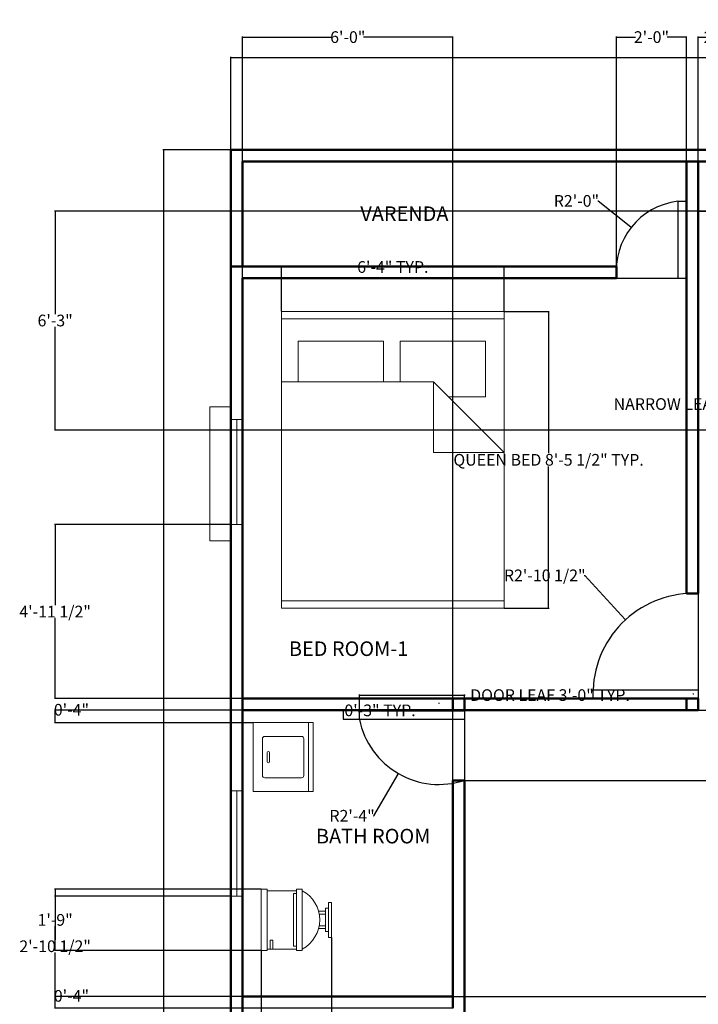
# Model space of a CAD drawing. Units: inches. Extents: x 749 to 1356, y 222 to 907.
# Tile 3 of 4: x 749 to 981, y 570 to 907. Entities that reach past the tile are written whole.
import ezdxf

# ---------------------------------------------------------------- set-up
doc = ezdxf.new("R2010")
doc.units = ezdxf.units.IN
doc.header["$MEASUREMENT"] = 0
for name, color, linetype, lineweight in [('A-ANNO-DIMS', 30, 'Continuous', 18), ('A-AREA-IDEN', 6, 'Continuous', 25), ('A-FLOR-CASE', 34, 'Continuous', 25), ('A-FLOR-FIXT', 9, 'Continuous', 18), ('A-GLAZ', 4, 'Continuous', 20), ('A-WALL', 7, 'Continuous', 50), ('DOOR', 4, 'Continuous', 25), ('FURNITURE', 32, 'Continuous', 18)]:
    doc.layers.add(name, color=color, linetype=linetype, lineweight=lineweight)
doc.styles.get("Standard").update_dxf_attribs({"font": 'arial.ttf'})
doc.dimstyles.get("Standard").update_dxf_attribs({"dimtxt": 4, "dimasz": 0.18, "dimexe": 0.18, "dimexo": 0.0625, "dimgap": 0.09, "dimtad": 0, "dimtih": 1, "dimtoh": 1, "dimdec": 0, "dimrnd": 6, "dimzin": 0, "dimdsep": 46, "dimlunit": 3, "dimtxsty": 'Standard', "dimcen": 0.09, "dimadec": 0, "dimazin": 0, "dimtfac": 1, "dimtdec": 0, "dimtofl": 0, "dimtmove": 0, "dimatfit": 3, "dimfxl": 1, "dimtolj": 1, "dimtzin": 0, "dimarcsym": 0})

# ---------------------------------------------------------------- blocks, each defined once
blk = doc.blocks.new('Toilet - Imperial')
for p, q in [((-10, 22), (-10, 12)), ((-10, 21), (-7, 21)), ((-7, 21), (-7, 20)), ((10, 12), (10, 22)), ((-7, 20), (-10, 20)), ((10.5, 12), (-10.5, 12)), ((-10.5, 10), (-10.5, 12)), ((9, 13), (-9, 13)), ((-9, 13), (-9, 12)), ((9, 12), (9, 13)), ((10.5, 12), (10.5, 10)), ((10.5, 10), (-10.5, 10)), ((-3, 4.4065), (-3, 2)), ((-2, 2), (-2, 4.1658)), ((2, 4.1658), (2, 2)), ((3, 2), (3, 4.4065)), ((4, 2), (-4, 2)), ((-4, 2), (-4, 1)), ((4, 1), (4, 2))]:
    blk.add_line(p, q)
for points in [[(10.5, 22), (10.5, 24), (-10.5, 24), (-10.5, 22)], [(6, 0), (6, 1), (-6, 1), (-6, 0)]]:
    blk.add_lwpolyline(points, close=True)
blk.add_arc((0, 15.3333), 11.3333, 208.0725, 331.9275)
blk = doc.blocks.new('QUEEN-00')
for p, q in [((-0.8475, -0.7751), (-0.8475, 0.7489)), ((0.6511, 0.7489), (0.6511, -0.2925)), ((1.0829, 0.7489), (1.0829, -0.7751)), ((0.9305, 0.6346), (0.6511, 0.6346)), ((0.9305, 0.0504), (0.9305, 0.6346)), ((0.6511, 0.0504), (0.9305, 0.0504)), ((0.9305, -0.0639), (0.6511, -0.0639)), ((0.9305, -0.6481), (0.9305, -0.0639)), ((0.1685, -0.7751), (0.6511, -0.2925)), ((0.1685, -0.2925), (0.1685, -0.7751)), ((0.6511, -0.2925), (0.1685, -0.2925)), ((0.5495, -0.3941), (0.5495, -0.6481)), ((0.5495, -0.6481), (0.9305, -0.6481))]:
    blk.add_line(p, q)
blk.add_lwpolyline([(-0.8983, -0.7751), (-0.8983, 0.7489), (1.1337, 0.7489), (1.1337, -0.7751)], close=True)
blk = doc.blocks.new('LAVAD-01')
for p, q in [((-0.322, 0.358), (-0.322, -0.392)), ((0.328, 0.358), (-0.322, 0.358)), ((-0.272, 0.358), (-0.272, -0.392)), ((0.328, -0.392), (0.328, 0.358)), ((-0.222, 0.183), (-0.222, -0.217)), ((0.203, 0.208), (-0.197, 0.208)), ((0.228, -0.217), (0.228, 0.183)), ((0.153, 0.033), (0.153, -0.067)), ((0.165, 0.046), (0.165, 0.046)), ((0.178, -0.067), (0.178, 0.033)), ((0.165, -0.079), (0.165, -0.079)), ((-0.197, -0.242), (0.203, -0.242)), ((-0.322, -0.392), (0.328, -0.392))]:
    blk.add_line(p, q)
for centre, radius, start, end in [((-0.197, 0.183), 0.025, 90, 180), ((0.203, 0.183), 0.025, 0, 90), ((0.165, 0.033), 0.0125, 90, 180), ((0.165, 0.033), 0.0125, 0, 90), ((0.165, -0.067), 0.0125, 180, 270), ((0.165, -0.067), 0.0125, 270, 360), ((-0.197, -0.217), 0.025, 180, 270), ((0.203, -0.217), 0.025, 270, 360)]:
    blk.add_arc(centre, radius, start, end)
blk = doc.blocks.new('*D129')
at = {"layer": 'A-ANNO-DIMS', "color": 0, "lineweight": -2, "transparency": 16777216}
for p, q in [((820.88, 858.33), (820.88, 894.09)), ((821.06, 893.91), (1057.31, 893.91)), ((1300.7, 893.91), (1064.44, 893.91)), ((1300.88, 862.33), (1300.88, 894.09))]:
    blk.add_line(p, q, dxfattribs=at)
at = {"layer": 'A-ANNO-DIMS', "color": 0, "transparency": 16777216}
for points in [[(821.06, 893.94), (821.06, 893.88), (820.88, 893.91)], [(1300.7, 893.94), (1300.7, 893.88), (1300.88, 893.91)]]:
    blk.add_solid(points, dxfattribs=at)
at = {"layer": 'Defpoints', "color": 0, "transparency": 16777216}
for p in [(1300.88, 893.91), (1300.88, 862.27), (820.88, 858.27)]:
    blk.add_point(p, dxfattribs=at)
at = {"layer": 'A-ANNO-DIMS', "color": 0, "transparency": 16777216, "insert": (1060.88, 893.91), "char_height": 4, "attachment_point": 5}
blk.add_mtext("\\A1;40'", dxfattribs=at)
blk = doc.blocks.new('*D130')
at = {"layer": 'A-ANNO-DIMS', "color": 0, "lineweight": -2, "transparency": 16777216}
for p, q in [((820.81, 862.27), (797.55, 862.27)), ((797.73, 862.09), (797.73, 564.4)), ((797.73, 262.45), (797.73, 560.13)), ((820.81, 262.27), (797.55, 262.27))]:
    blk.add_line(p, q, dxfattribs=at)
at = {"layer": 'A-ANNO-DIMS', "color": 0, "transparency": 16777216}
for points in [[(797.7, 862.09), (797.76, 862.09), (797.73, 862.27)], [(797.7, 262.45), (797.76, 262.45), (797.73, 262.27)]]:
    blk.add_solid(points, dxfattribs=at)
at = {"layer": 'Defpoints', "color": 0, "transparency": 16777216}
for p in [(820.88, 862.27), (797.73, 262.27), (820.88, 262.27)]:
    blk.add_point(p, dxfattribs=at)
at = {"layer": 'A-ANNO-DIMS', "color": 0, "transparency": 16777216, "insert": (797.73, 562.27), "char_height": 4, "attachment_point": 5}
blk.add_mtext("\\A1;50'", dxfattribs=at)
blk = doc.blocks.new('WIN-36IN')
blk.add_lwpolyline([(0, 0), (0, 36), (4, 36), (4, 0)], close=True)
blk.add_lwpolyline([(4, 0), (2.02, 0), (2.02, 36)])
blk = doc.blocks.new('DOOR-LEAF-36IN')
blk.add_lwpolyline([(0, 3), (36, 3), (36, 0), (0, 0)], close=True)
blk = doc.blocks.new('*D137')
at = {"layer": 'A-ANNO-DIMS', "color": 0, "lineweight": -2, "transparency": 16777216}
for p, q in [((864.87, 670.13), (864.87, 675.65)), ((865.05, 675.47), (900.69, 675.47)), ((900.87, 670.13), (900.87, 675.65)), ((900.87, 675.47), (901.05, 675.47))]:
    blk.add_line(p, q, dxfattribs=at)
at = {"layer": 'A-ANNO-DIMS', "color": 0, "transparency": 16777216}
for points in [[(865.05, 675.5), (865.05, 675.44), (864.87, 675.47)], [(900.69, 675.5), (900.69, 675.44), (900.87, 675.47)]]:
    blk.add_solid(points, dxfattribs=at)
at = {"layer": 'Defpoints', "color": 0, "transparency": 16777216}
for p in [(900.87, 675.47), (864.87, 670.07), (900.87, 670.07)]:
    blk.add_point(p, dxfattribs=at)
at = {"layer": 'A-ANNO-DIMS', "color": 0, "transparency": 16777216, "insert": (930.15, 675.47), "char_height": 4, "attachment_point": 5}
blk.add_mtext('\\A1;DOOR LEAF 3\'-0" TYP.', dxfattribs=at)
blk = doc.blocks.new('*D138')
at = {"layer": 'A-ANNO-DIMS', "color": 0, "lineweight": -2, "transparency": 16777216}
for p, q in [((864.81, 670.07), (859.29, 670.07)), ((859.47, 670.07), (859.47, 670.25)), ((859.47, 670.25), (859.65, 670.25)), ((859.47, 667.25), (859.47, 669.89)), ((864.81, 667.07), (859.29, 667.07))]:
    blk.add_line(p, q, dxfattribs=at)
at = {"layer": 'A-ANNO-DIMS', "color": 0, "transparency": 16777216}
for points in [[(859.44, 669.89), (859.5, 669.89), (859.47, 670.07)], [(859.44, 667.25), (859.5, 667.25), (859.47, 667.07)]]:
    blk.add_solid(points, dxfattribs=at)
at = {"layer": 'Defpoints', "color": 0, "transparency": 16777216}
for p in [(859.47, 670.07), (864.87, 670.07), (864.87, 667.07)]:
    blk.add_point(p, dxfattribs=at)
at = {"layer": 'A-ANNO-DIMS', "color": 0, "transparency": 16777216, "insert": (871.93, 670.25), "char_height": 4, "attachment_point": 5}
blk.add_mtext('\\A1;0\'-3" TYP.', dxfattribs=at)
blk = doc.blocks.new('*D141')
at = {"layer": 'A-ANNO-DIMS', "color": 0, "lineweight": -2, "transparency": 16777216}
for p, q in [((984.05, 787.99), (988.01, 787.99)), ((987.83, 787.81), (987.83, 777.32)), ((987.83, 762.5), (987.83, 773)), ((984.05, 762.32), (988.01, 762.32))]:
    blk.add_line(p, q, dxfattribs=at)
at = {"layer": 'A-ANNO-DIMS', "color": 0, "transparency": 16777216}
for points in [[(987.8, 787.81), (987.86, 787.81), (987.83, 787.99)], [(987.8, 762.5), (987.86, 762.5), (987.83, 762.32)]]:
    blk.add_solid(points, dxfattribs=at)
at = {"layer": 'Defpoints', "color": 0, "transparency": 16777216}
for p in [(983.98, 787.99), (987.83, 787.99), (983.98, 762.32)]:
    blk.add_point(p, dxfattribs=at)
at = {"layer": 'A-ANNO-DIMS', "color": 0, "transparency": 16777216, "insert": (987.83, 775.16), "char_height": 4, "attachment_point": 5}
blk.add_mtext('\\A1;NARROW LEAF 2\'-1 1/2" TYP.', dxfattribs=at)
blk = doc.blocks.new('*D147')
at = {"layer": 'A-ANNO-DIMS', "color": 0, "lineweight": -2, "transparency": 16777216}
for p, q in [((914.47, 806.86), (929.83, 806.86)), ((929.65, 806.68), (929.65, 758.35)), ((929.65, 705.44), (929.65, 753.78)), ((914.47, 705.26), (929.83, 705.26))]:
    blk.add_line(p, q, dxfattribs=at)
at = {"layer": 'A-ANNO-DIMS', "color": 0, "transparency": 16777216}
for points in [[(929.62, 806.68), (929.68, 806.68), (929.65, 806.86)], [(929.62, 705.44), (929.68, 705.44), (929.65, 705.26)]]:
    blk.add_solid(points, dxfattribs=at)
at = {"layer": 'Defpoints', "color": 0, "transparency": 16777216}
for p in [(914.41, 806.86), (929.65, 806.86), (914.41, 705.26)]:
    blk.add_point(p, dxfattribs=at)
at = {"layer": 'A-ANNO-DIMS', "color": 0, "transparency": 16777216, "insert": (929.65, 756.06), "char_height": 4, "attachment_point": 5}
blk.add_mtext('\\A1;QUEEN BED 8\'-5 1/2" TYP.', dxfattribs=at)
blk = doc.blocks.new('*D148')
at = {"layer": 'A-ANNO-DIMS', "color": 0, "lineweight": -2, "transparency": 16777216}
for p, q in [((838.21, 806.93), (838.21, 822.28)), ((838.39, 822.1), (864.02, 822.1)), ((914.23, 822.1), (888.6, 822.1)), ((914.41, 806.93), (914.41, 822.28))]:
    blk.add_line(p, q, dxfattribs=at)
at = {"layer": 'A-ANNO-DIMS', "color": 0, "transparency": 16777216}
for points in [[(838.39, 822.13), (838.39, 822.07), (838.21, 822.1)], [(914.23, 822.13), (914.23, 822.07), (914.41, 822.1)]]:
    blk.add_solid(points, dxfattribs=at)
at = {"layer": 'Defpoints', "color": 0, "transparency": 16777216}
for p in [(838.21, 822.1), (838.21, 806.86), (914.41, 806.86)]:
    blk.add_point(p, dxfattribs=at)
at = {"layer": 'A-ANNO-DIMS', "color": 0, "transparency": 16777216, "insert": (876.31, 822.1), "char_height": 4, "attachment_point": 5}
blk.add_mtext('\\A1;6\'-4" TYP.', dxfattribs=at)
blk = doc.blocks.new('*D167')
at = {"layer": 'A-ANNO-DIMS', "color": 0, "lineweight": -2, "transparency": 16777216}
for p, q in [((820.83, 733.87), (760.48, 733.87)), ((760.66, 733.69), (760.66, 706.22)), ((760.66, 674.45), (760.66, 701.91)), ((824.81, 674.27), (760.48, 674.27))]:
    blk.add_line(p, q, dxfattribs=at)
at = {"layer": 'A-ANNO-DIMS', "color": 0, "transparency": 16777216}
for points in [[(760.63, 733.69), (760.69, 733.69), (760.66, 733.87)], [(760.63, 674.45), (760.69, 674.45), (760.66, 674.27)]]:
    blk.add_solid(points, dxfattribs=at)
at = {"layer": 'Defpoints', "color": 0, "transparency": 16777216}
for p in [(760.66, 733.87), (820.89, 733.87), (824.88, 674.27)]:
    blk.add_point(p, dxfattribs=at)
at = {"layer": 'A-ANNO-DIMS', "color": 0, "transparency": 16777216, "insert": (760.66, 704.07), "char_height": 4, "attachment_point": 5}
blk.add_mtext('\\A1;4\'-11 1/2"', dxfattribs=at)
blk = doc.blocks.new('*D169')
at = {"layer": 'A-ANNO-DIMS', "color": 0, "lineweight": -2, "transparency": 16777216}
for p, q in [((980.88, 858.33), (980.88, 901.02)), ((981.06, 900.84), (997, 900.84)), ((1033.23, 900.84), (1017.29, 900.84)), ((1033.41, 858.31), (1033.41, 901.02))]:
    blk.add_line(p, q, dxfattribs=at)
at = {"layer": 'A-ANNO-DIMS', "color": 0, "transparency": 16777216}
for points in [[(981.06, 900.87), (981.06, 900.81), (980.88, 900.84)], [(1033.23, 900.87), (1033.23, 900.81), (1033.41, 900.84)]]:
    blk.add_solid(points, dxfattribs=at)
at = {"layer": 'Defpoints', "color": 0, "transparency": 16777216}
for p in [(1033.41, 900.84), (980.88, 858.27), (1033.41, 858.25)]:
    blk.add_point(p, dxfattribs=at)
at = {"layer": 'A-ANNO-DIMS', "color": 0, "transparency": 16777216, "insert": (1007.14, 900.84), "char_height": 4, "attachment_point": 5}
blk.add_mtext('\\A1;4\'-4 1/2"', dxfattribs=at)
blk = doc.blocks.new('*D171')
at = {"layer": 'A-ANNO-DIMS', "color": 0, "lineweight": -2, "transparency": 16777216}
for p, q in [((820.81, 606.63), (760.48, 606.63)), ((760.66, 606.45), (760.66, 591.61)), ((760.66, 572.45), (760.66, 587.29)), ((824.81, 572.27), (760.48, 572.27))]:
    blk.add_line(p, q, dxfattribs=at)
at = {"layer": 'A-ANNO-DIMS', "color": 0, "transparency": 16777216}
for points in [[(760.63, 606.45), (760.69, 606.45), (760.66, 606.63)], [(760.63, 572.45), (760.69, 572.45), (760.66, 572.27)]]:
    blk.add_solid(points, dxfattribs=at)
at = {"layer": 'Defpoints', "color": 0, "transparency": 16777216}
for p in [(760.66, 606.63), (820.87, 606.63), (824.88, 572.27)]:
    blk.add_point(p, dxfattribs=at)
at = {"layer": 'A-ANNO-DIMS', "color": 0, "transparency": 16777216, "insert": (760.66, 589.45), "char_height": 4, "attachment_point": 5}
blk.add_mtext('\\A1;2\'-10 1/2"', dxfattribs=at)
blk = doc.blocks.new('*D172')
at = {"layer": 'A-ANNO-DIMS', "color": 0, "lineweight": -2, "transparency": 16777216}
for p, q in [((824.88, 572.33), (824.88, 901.02)), ((825.06, 900.84), (855.46, 900.84)), ((896.7, 900.84), (866.29, 900.84)), ((896.88, 572.33), (896.88, 901.02))]:
    blk.add_line(p, q, dxfattribs=at)
at = {"layer": 'A-ANNO-DIMS', "color": 0, "transparency": 16777216}
for points in [[(825.06, 900.87), (825.06, 900.81), (824.88, 900.84)], [(896.7, 900.87), (896.7, 900.81), (896.88, 900.84)]]:
    blk.add_solid(points, dxfattribs=at)
at = {"layer": 'Defpoints', "color": 0, "transparency": 16777216}
for p in [(896.88, 900.84), (824.88, 572.27), (896.88, 572.27)]:
    blk.add_point(p, dxfattribs=at)
at = {"layer": 'A-ANNO-DIMS', "color": 0, "transparency": 16777216, "insert": (860.88, 900.84), "char_height": 4, "attachment_point": 5}
blk.add_mtext('\\A1;6\'-0"', dxfattribs=at)
blk = doc.blocks.new('*D174')
at = {"layer": 'A-ANNO-DIMS', "color": 0, "lineweight": -2, "transparency": 16777216}
for p, q in [((900.94, 646.27), (1340.58, 646.27)), ((1340.4, 646.09), (1340.4, 611.4)), ((1340.4, 572.45), (1340.4, 607.13)), ((896.94, 572.27), (1340.58, 572.27))]:
    blk.add_line(p, q, dxfattribs=at)
at = {"layer": 'A-ANNO-DIMS', "color": 0, "transparency": 16777216}
for points in [[(1340.37, 646.09), (1340.43, 646.09), (1340.4, 646.27)], [(1340.37, 572.45), (1340.43, 572.45), (1340.4, 572.27)]]:
    blk.add_solid(points, dxfattribs=at)
at = {"layer": 'Defpoints', "color": 0, "transparency": 16777216}
for p in [(900.88, 646.27), (1340.4, 646.27), (896.88, 572.27)]:
    blk.add_point(p, dxfattribs=at)
at = {"layer": 'A-ANNO-DIMS', "color": 0, "transparency": 16777216, "insert": (1340.4, 609.27), "char_height": 4, "attachment_point": 5}
blk.add_mtext('\\A1;6\'-2"', dxfattribs=at)
blk = doc.blocks.new('*D175')
at = {"layer": 'A-ANNO-DIMS', "color": 0, "lineweight": -2, "transparency": 16777216}
for p, q in [((900.94, 670.27), (1340.58, 670.27)), ((1340.4, 670.09), (1340.4, 660.4)), ((1340.4, 646.45), (1340.4, 656.13)), ((900.94, 646.27), (1340.58, 646.27))]:
    blk.add_line(p, q, dxfattribs=at)
at = {"layer": 'A-ANNO-DIMS', "color": 0, "transparency": 16777216}
for points in [[(1340.37, 670.09), (1340.43, 670.09), (1340.4, 670.27)], [(1340.37, 646.45), (1340.43, 646.45), (1340.4, 646.27)]]:
    blk.add_solid(points, dxfattribs=at)
at = {"layer": 'Defpoints', "color": 0, "transparency": 16777216}
for p in [(900.88, 670.27), (1340.4, 670.27), (900.88, 646.27)]:
    blk.add_point(p, dxfattribs=at)
at = {"layer": 'A-ANNO-DIMS', "color": 0, "transparency": 16777216, "insert": (1340.4, 658.27), "char_height": 4, "attachment_point": 5}
blk.add_mtext('\\A1;2\'-0"', dxfattribs=at)
blk = doc.blocks.new('*D177')
at = {"layer": 'A-ANNO-DIMS', "color": 0, "lineweight": -2, "transparency": 16777216}
for p, q in [((855.27, 592.42), (855.27, 224.8)), ((831.27, 587.92), (831.27, 224.8)), ((831.45, 224.98), (837.83, 224.98)), ((855.09, 224.98), (848.71, 224.98))]:
    blk.add_line(p, q, dxfattribs=at)
at = {"layer": 'A-ANNO-DIMS', "color": 0, "transparency": 16777216}
for points in [[(831.45, 225.01), (831.45, 224.95), (831.27, 224.98)], [(855.09, 225.01), (855.09, 224.95), (855.27, 224.98)]]:
    blk.add_solid(points, dxfattribs=at)
at = {"layer": 'Defpoints', "color": 0, "transparency": 16777216}
for p in [(855.27, 592.48), (831.27, 587.98), (855.27, 224.98)]:
    blk.add_point(p, dxfattribs=at)
at = {"layer": 'A-ANNO-DIMS', "color": 0, "transparency": 16777216, "insert": (843.27, 224.98), "char_height": 4, "attachment_point": 5}
blk.add_mtext('\\A1;2\'-0"', dxfattribs=at)
blk = doc.blocks.new('*D178')
at = {"layer": 'A-ANNO-DIMS', "color": 0, "lineweight": -2, "transparency": 16777216}
for p, q in [((831.21, 608.98), (760.48, 608.98)), ((760.66, 608.8), (760.66, 600.62)), ((760.66, 588.16), (760.66, 596.35)), ((831.21, 587.98), (760.48, 587.98))]:
    blk.add_line(p, q, dxfattribs=at)
at = {"layer": 'A-ANNO-DIMS', "color": 0, "transparency": 16777216}
for points in [[(760.63, 608.8), (760.69, 608.8), (760.66, 608.98)], [(760.63, 588.16), (760.69, 588.16), (760.66, 587.98)]]:
    blk.add_solid(points, dxfattribs=at)
at = {"layer": 'Defpoints', "color": 0, "transparency": 16777216}
for p in [(760.66, 608.98), (831.27, 608.98), (831.27, 587.98)]:
    blk.add_point(p, dxfattribs=at)
at = {"layer": 'A-ANNO-DIMS', "color": 0, "transparency": 16777216, "insert": (760.66, 598.48), "char_height": 4, "attachment_point": 5}
blk.add_mtext('\\A1;1\'-9"', dxfattribs=at)
blk = doc.blocks.new('*D179')
at = {"layer": 'A-ANNO-DIMS', "color": 0, "lineweight": -2, "transparency": 16777216}
for p, q in [((1112.81, 841.27), (760.48, 841.27)), ((760.66, 841.09), (760.66, 805.9)), ((760.66, 766.45), (760.66, 801.63)), ((1112.81, 766.27), (760.48, 766.27))]:
    blk.add_line(p, q, dxfattribs=at)
at = {"layer": 'A-ANNO-DIMS', "color": 0, "transparency": 16777216}
for points in [[(760.63, 841.09), (760.69, 841.09), (760.66, 841.27)], [(760.63, 766.45), (760.69, 766.45), (760.66, 766.27)]]:
    blk.add_solid(points, dxfattribs=at)
at = {"layer": 'Defpoints', "color": 0, "transparency": 16777216}
for p in [(760.66, 841.27), (1112.88, 841.27), (1112.88, 766.27)]:
    blk.add_point(p, dxfattribs=at)
at = {"layer": 'A-ANNO-DIMS', "color": 0, "transparency": 16777216, "insert": (760.66, 803.77), "char_height": 4, "attachment_point": 5}
blk.add_mtext('\\A1;6\'-3"', dxfattribs=at)
blk = doc.blocks.new('*D182')
at = {"layer": 'A-ANNO-DIMS', "color": 0, "lineweight": -2, "transparency": 16777216}
for p, q in [((980.94, 858.27), (1340.58, 858.27)), ((1340.4, 858.09), (1340.4, 851.9)), ((1340.4, 841.45), (1340.4, 847.63)), ((980.94, 841.27), (1340.58, 841.27))]:
    blk.add_line(p, q, dxfattribs=at)
at = {"layer": 'A-ANNO-DIMS', "color": 0, "transparency": 16777216}
for points in [[(1340.37, 858.09), (1340.43, 858.09), (1340.4, 858.27)], [(1340.37, 841.45), (1340.43, 841.45), (1340.4, 841.27)]]:
    blk.add_solid(points, dxfattribs=at)
at = {"layer": 'Defpoints', "color": 0, "transparency": 16777216}
for p in [(980.88, 858.27), (1340.4, 858.27), (980.88, 841.27)]:
    blk.add_point(p, dxfattribs=at)
at = {"layer": 'A-ANNO-DIMS', "color": 0, "transparency": 16777216, "insert": (1340.4, 849.77), "char_height": 4, "attachment_point": 5}
blk.add_mtext('\\A1;1\'-5"', dxfattribs=at)
blk = doc.blocks.new('*D183')
at = {"layer": 'A-ANNO-DIMS', "color": 0, "lineweight": -2, "transparency": 16777216}
for p, q in [((896.81, 572.27), (760.48, 572.27)), ((760.66, 572.27), (760.66, 572.45)), ((760.66, 572.45), (760.84, 572.45)), ((760.66, 568.45), (760.66, 572.09)), ((896.81, 568.27), (760.48, 568.27))]:
    blk.add_line(p, q, dxfattribs=at)
at = {"layer": 'A-ANNO-DIMS', "color": 0, "transparency": 16777216}
for points in [[(760.63, 572.09), (760.69, 572.09), (760.66, 572.27)], [(760.63, 568.45), (760.69, 568.45), (760.66, 568.27)]]:
    blk.add_solid(points, dxfattribs=at)
at = {"layer": 'Defpoints', "color": 0, "transparency": 16777216}
for p in [(760.66, 572.27), (896.88, 572.27), (896.88, 568.27)]:
    blk.add_point(p, dxfattribs=at)
at = {"layer": 'A-ANNO-DIMS', "color": 0, "transparency": 16777216, "insert": (766.25, 572.45), "char_height": 4, "attachment_point": 5}
blk.add_mtext('\\A1;0\'-4"', dxfattribs=at)
blk = doc.blocks.new('*D184')
at = {"layer": 'A-ANNO-DIMS', "color": 0, "lineweight": -2, "transparency": 16777216}
for p, q in [((980.88, 841.33), (980.88, 901.02)), ((981.06, 900.84), (983.41, 900.84)), ((1005.96, 900.84), (1003.61, 900.84)), ((1006.14, 842.02), (1006.14, 901.02))]:
    blk.add_line(p, q, dxfattribs=at)
at = {"layer": 'A-ANNO-DIMS', "color": 0, "transparency": 16777216}
for points in [[(981.06, 900.87), (981.06, 900.81), (980.88, 900.84)], [(1005.96, 900.87), (1005.96, 900.81), (1006.14, 900.84)]]:
    blk.add_solid(points, dxfattribs=at)
at = {"layer": 'Defpoints', "color": 0, "transparency": 16777216}
for p in [(1006.14, 900.84), (980.88, 841.27), (1006.14, 841.95)]:
    blk.add_point(p, dxfattribs=at)
at = {"layer": 'A-ANNO-DIMS', "color": 0, "transparency": 16777216, "insert": (993.51, 900.84), "char_height": 4, "attachment_point": 5}
blk.add_mtext('\\A1;2\'-1 1/2"', dxfattribs=at)
blk = doc.blocks.new('*D186')
at = {"layer": 'A-ANNO-DIMS', "color": 0, "lineweight": -2, "transparency": 16777216}
for p, q in [((952.88, 822.33), (952.88, 901.02)), ((953.06, 900.84), (959.44, 900.84)), ((976.7, 900.84), (970.32, 900.84)), ((976.88, 818.33), (976.88, 901.02))]:
    blk.add_line(p, q, dxfattribs=at)
at = {"layer": 'A-ANNO-DIMS', "color": 0, "transparency": 16777216}
for points in [[(953.06, 900.87), (953.06, 900.81), (952.88, 900.84)], [(976.7, 900.87), (976.7, 900.81), (976.88, 900.84)]]:
    blk.add_solid(points, dxfattribs=at)
at = {"layer": 'Defpoints', "color": 0, "transparency": 16777216}
for p in [(976.88, 900.84), (952.88, 822.27), (976.88, 818.27)]:
    blk.add_point(p, dxfattribs=at)
at = {"layer": 'A-ANNO-DIMS', "color": 0, "transparency": 16777216, "insert": (964.88, 900.84), "char_height": 4, "attachment_point": 5}
blk.add_mtext('\\A1;2\'-0"', dxfattribs=at)
blk = doc.blocks.new('*D188')
at = {"layer": 'A-ANNO-DIMS', "color": 0, "lineweight": -2, "transparency": 16777216}
for p, q in [((824.81, 670.27), (760.48, 670.27)), ((760.66, 670.27), (760.66, 670.45)), ((760.66, 670.45), (760.84, 670.45)), ((760.66, 666.21), (760.66, 670.09)), ((828.45, 666.03), (760.48, 666.03))]:
    blk.add_line(p, q, dxfattribs=at)
at = {"layer": 'A-ANNO-DIMS', "color": 0, "transparency": 16777216}
for points in [[(760.63, 670.09), (760.69, 670.09), (760.66, 670.27)], [(760.63, 666.21), (760.69, 666.21), (760.66, 666.03)]]:
    blk.add_solid(points, dxfattribs=at)
at = {"layer": 'Defpoints', "color": 0, "transparency": 16777216}
for p in [(760.66, 670.27), (824.88, 670.27), (828.51, 666.03)]:
    blk.add_point(p, dxfattribs=at)
at = {"layer": 'A-ANNO-DIMS', "color": 0, "transparency": 16777216, "insert": (766.25, 670.45), "char_height": 4, "attachment_point": 5}
blk.add_mtext('\\A1;0\'-4"', dxfattribs=at)
blk = doc.blocks.new('*D197')
at = {"layer": 'A-ANNO-DIMS', "color": 0, "lineweight": -2, "transparency": 16777216}
for p, q in [((941.88, 716.48), (942.06, 716.48)), ((942.06, 716.48), (955.88, 701.39)), ((979.16, 675.9), (979.34, 675.9)), ((979.25, 675.81), (979.25, 675.99))]:
    blk.add_line(p, q, dxfattribs=at)
at = {"layer": 'A-ANNO-DIMS', "color": 0, "transparency": 16777216}
blk.add_solid([(955.91, 701.42), (955.86, 701.37), (956.01, 701.26)], dxfattribs=at)
at = {"layer": 'Defpoints', "color": 0, "transparency": 16777216}
for p in [(956.01, 701.26), (979.25, 675.9)]:
    blk.add_point(p, dxfattribs=at)
at = {"layer": 'A-ANNO-DIMS', "color": 0, "transparency": 16777216, "insert": (928.34, 716.48), "char_height": 4, "attachment_point": 5}
blk.add_mtext('\\A1;R2\'-10 1/2"', dxfattribs=at)
blk = doc.blocks.new('*D199')
at = {"layer": 'A-ANNO-DIMS', "color": 0, "lineweight": -2, "transparency": 16777216}
for p, q in [((892.05, 672.72), (892.23, 672.72)), ((892.14, 672.63), (892.14, 672.81)), ((869.85, 634.13), (878.12, 648.44)), ((869.67, 634.13), (869.85, 634.13))]:
    blk.add_line(p, q, dxfattribs=at)
at = {"layer": 'A-ANNO-DIMS', "color": 0, "transparency": 16777216}
blk.add_solid([(878.09, 648.46), (878.15, 648.43), (878.21, 648.6)], dxfattribs=at)
at = {"layer": 'Defpoints', "color": 0, "transparency": 16777216}
for p in [(892.14, 672.72), (878.21, 648.6)]:
    blk.add_point(p, dxfattribs=at)
at = {"layer": 'A-ANNO-DIMS', "color": 0, "transparency": 16777216, "insert": (862.35, 634.13), "char_height": 4, "attachment_point": 5}
blk.add_mtext('\\A1;R2\'-4"', dxfattribs=at)
blk = doc.blocks.new('*D200')
at = {"layer": 'A-ANNO-DIMS', "color": 0, "lineweight": -2, "transparency": 16777216}
for p, q in [((946.51, 844.74), (946.69, 844.74)), ((946.69, 844.74), (957.87, 835.83)), ((976.79, 820.69), (976.97, 820.69)), ((976.88, 820.6), (976.88, 820.78))]:
    blk.add_line(p, q, dxfattribs=at)
at = {"layer": 'A-ANNO-DIMS', "color": 0, "transparency": 16777216}
blk.add_solid([(957.89, 835.85), (957.85, 835.81), (958.01, 835.72)], dxfattribs=at)
at = {"layer": 'Defpoints', "color": 0, "transparency": 16777216}
for p in [(958.01, 835.72), (976.88, 820.69)]:
    blk.add_point(p, dxfattribs=at)
at = {"layer": 'A-ANNO-DIMS', "color": 0, "transparency": 16777216, "insert": (939.19, 844.74), "char_height": 4, "attachment_point": 5}
blk.add_mtext('\\A1;R2\'-0"', dxfattribs=at)

msp = doc.modelspace()

# ---------------------------------------------------------------- linework, layer by layer
at = {"layer": 'A-FLOR-CASE'}
msp.add_line((1112.88, 841.27), (980.88, 841.27), dxfattribs=at)
at = {"layer": 'A-GLAZ'}
for p, q in [((820.88, 774.15), (813.64, 774.15)), ((813.64, 774.15), (813.64, 728.35)), ((813.64, 728.35), (820.88, 728.35))]:
    msp.add_line(p, q, dxfattribs=at)
at = {"layer": 'A-WALL'}
for p, q in [((1300.88, 862.27), (820.88, 862.27)), ((820.88, 862.27), (820.88, 262.27)), ((1296.88, 858.27), (824.88, 858.27)), ((824.88, 858.27), (824.88, 822.27)), ((976.88, 858.27), (976.88, 710.27)), ((980.88, 858.27), (980.88, 710.27)), ((976.88, 842.16), (976.88, 818.27)), ((952.88, 822.27), (820.88, 822.27)), ((952.88, 822.27), (952.88, 818.27)), ((824.88, 818.27), (824.88, 470.27)), ((952.88, 818.27), (824.88, 818.27)), ((980.88, 710.27), (976.88, 710.27)), ((980.88, 674.27), (824.88, 674.27)), ((896.88, 674.27), (896.88, 670.27)), ((900.88, 674.27), (900.88, 670.27)), ((976.88, 674.27), (976.88, 670.27)), ((980.88, 674.27), (980.88, 670.27)), ((980.88, 670.27), (824.88, 670.27)), ((900.88, 646.27), (896.88, 646.27)), ((896.88, 646.27), (896.88, 572.27)), ((900.88, 646.27), (900.88, 466.27)), ((896.88, 572.27), (824.88, 572.27)), ((896.88, 572.27), (896.88, 568.27))]:
    msp.add_line(p, q, dxfattribs=at)
at = {"layer": 'DOOR'}
for p, q in [((973.88, 844.62), (976.88, 844.62)), ((976.88, 844.62), (976.88, 844.62)), ((952.88, 818.27), (973.88, 818.27)), ((980.88, 710.27), (980.88, 677.27)), ((900.87, 667.07), (900.87, 646.27))]:
    msp.add_line(p, q, dxfattribs=at)
msp.add_lwpolyline([(973.88, 844.62), (973.88, 818.27), (976.88, 818.27), (976.88, 844.62)], dxfattribs=at)
for centre, radius, start, end in [((976.88, 820.69), 24.12, 97.1417, 185.7569), ((979.25, 675.9), 34.4, 87.2961, 177.7248), ((892.14, 672.72), 27.85, 191.6941, 288.2734)]:
    msp.add_arc(centre, radius, start, end, dxfattribs=at)

# ---------------------------------------------------------------- block references
at = {"layer": 'A-FLOR-FIXT', "xscale": 31.49606299212599, "yscale": 31.49606299212599, "zscale": 31.49606299212599, "rotation": 180}
msp.add_blockref('LAVAD-01', (838.84, 653.7), dxfattribs=at)
at = {"layer": 'A-FLOR-FIXT', "rotation": 90}
msp.add_blockref('Toilet - Imperial', (855.27, 598.48), dxfattribs=at)
at = {"layer": 'A-GLAZ'}
for p in [(820.9, 733.87), (820.87, 606.63)]:
    msp.add_blockref('WIN-36IN', p, dxfattribs=at)
at = {"layer": 'DOOR'}
for p in [(944.88, 674.27), (864.87, 667.07)]:
    msp.add_blockref('DOOR-LEAF-36IN', p, dxfattribs=at)
at = {"layer": 'FURNITURE', "xscale": 49.9999999999977, "yscale": 49.9999999999977, "zscale": 49.9999999999977, "rotation": 90}
msp.add_blockref('QUEEN-00', (875.65, 750.18), dxfattribs=at)

# ---------------------------------------------------------------- texts
at = {"layer": 'A-AREA-IDEN', "char_height": 5, "attachment_point": 1}
for s, insert in [('VARENDA', (865.18, 842.86)), ('BED ROOM-1', (840.73, 693.87)), ('BATH ROOM', (849.98, 629.67))]:
    msp.add_mtext_dynamic_manual_height_columns(s, width=49.3334, gutter_width=1, heights=[0], dxfattribs=dict(at, insert=insert))

# ---------------------------------------------------------------- dimensions: what is measured, and where the dimension line sits
at = {"layer": 'A-ANNO-DIMS'}
for base, p1, p2, override, picture, middle in [((1033.41, 900.84), (980.88, 858.27), (1033.41, 858.25), {"dimdec": 1, "dimlfac": 1, "dimrnd": 0, "dimzin": 1, "dimdsep": 46, "dimlunit": 4, "dimfrac": 2}, '*D169', (1007.14, 900.84)), ((1006.14, 900.84), (980.88, 841.27), (1006.14, 841.95), {"dimdec": 1, "dimlfac": 1, "dimrnd": 0, "dimzin": 1, "dimdsep": 46, "dimlunit": 4, "dimfrac": 2}, '*D184', (993.51, 900.84)), ((896.88, 900.84), (824.88, 572.27), (896.88, 572.27), {"dimdec": 1, "dimlfac": 1, "dimrnd": 0, "dimzin": 1, "dimdsep": 46, "dimlunit": 4, "dimfrac": 2}, '*D172', (860.88, 900.84)), ((976.88, 900.84), (952.88, 822.27), (976.88, 818.27), {"dimdec": 1, "dimlfac": 1, "dimrnd": 0, "dimzin": 1, "dimdsep": 46, "dimlunit": 4, "dimfrac": 2}, '*D186', (964.88, 900.84)), ((1300.88, 893.91), (820.88, 858.27), (1300.88, 862.27), {"dimclrd": 0, "dimclre": 0, "dimclrt": 0}, '*D129', (1060.88, 893.91)), ((855.27, 224.98), (831.27, 587.98), (855.27, 592.48), {"dimdec": 1, "dimlfac": 1, "dimrnd": 0, "dimzin": 1, "dimdsep": 46, "dimlunit": 4, "dimfrac": 2}, '*D177', (843.27, 224.98))]:
    dim = msp.add_linear_dim(base=base, p1=p1, p2=p2, dimstyle='Standard', override=override, dxfattribs=at)
    dim.commit()
    dim.dimension.update_dxf_attribs({"geometry": picture, "text_midpoint": middle})
for base, p1, p2, override, picture, middle in [((797.73, 262.27), (820.88, 862.27), (820.88, 262.27), {"dimclrd": 0, "dimclre": 0, "dimclrt": 0}, '*D130', (797.73, 562.27)), ((1340.4, 858.27), (980.88, 841.27), (980.88, 858.27), {"dimdec": 1, "dimlfac": 1, "dimrnd": 0, "dimzin": 1, "dimdsep": 46, "dimlunit": 4, "dimfrac": 2}, '*D182', (1340.4, 849.77)), ((760.66, 841.27), (1112.88, 766.27), (1112.88, 841.27), {"dimdec": 1, "dimlfac": 1, "dimrnd": 0, "dimzin": 1, "dimdsep": 46, "dimlunit": 4, "dimfrac": 2}, '*D179', (760.66, 803.77)), ((760.66, 733.87), (824.88, 674.27), (820.89, 733.87), {"dimdec": 1, "dimlfac": 1, "dimrnd": 0, "dimzin": 1, "dimdsep": 46, "dimlunit": 4, "dimfrac": 2}, '*D167', (760.66, 704.07)), ((760.66, 670.27), (828.51, 666.03), (824.88, 670.27), {"dimdec": 1, "dimlfac": 1, "dimrnd": 0, "dimzin": 1, "dimdsep": 46, "dimlunit": 4, "dimfrac": 2}, '*D188', (766.25, 670.45)), ((1340.4, 670.27), (900.88, 646.27), (900.88, 670.27), {"dimdec": 1, "dimlfac": 1, "dimrnd": 0, "dimzin": 1, "dimdsep": 46, "dimlunit": 4, "dimfrac": 2}, '*D175', (1340.4, 658.27)), ((1340.4, 646.27), (896.88, 572.27), (900.88, 646.27), {"dimdec": 1, "dimlfac": 1, "dimrnd": 0, "dimzin": 1, "dimdsep": 46, "dimlunit": 4, "dimfrac": 2}, '*D174', (1340.4, 609.27)), ((760.66, 608.98), (831.27, 587.98), (831.27, 608.98), {"dimdec": 1, "dimlfac": 1, "dimrnd": 0, "dimzin": 1, "dimdsep": 46, "dimlunit": 4, "dimfrac": 2}, '*D178', (760.66, 598.48)), ((760.66, 606.63), (824.88, 572.27), (820.87, 606.63), {"dimdec": 1, "dimlfac": 1, "dimrnd": 0, "dimzin": 1, "dimdsep": 46, "dimlunit": 4, "dimfrac": 2}, '*D171', (760.66, 589.45)), ((760.66, 572.27), (896.88, 568.27), (896.88, 572.27), {"dimdec": 1, "dimlfac": 1, "dimrnd": 0, "dimzin": 1, "dimdsep": 46, "dimlunit": 4, "dimfrac": 2}, '*D183', (766.25, 572.45))]:
    dim = msp.add_linear_dim(base=base, p1=p1, p2=p2, angle=90, dimstyle='Standard', override=override, dxfattribs=at)
    dim.commit()
    dim.dimension.update_dxf_attribs({"geometry": picture, "text_midpoint": middle})
for center, mpoint, picture, middle in [((976.88, 820.69), (958.01, 835.72), '*D200', (939.19, 844.74)), ((979.25, 675.9), (956.01, 701.26), '*D197', (928.34, 716.48)), ((892.14, 672.72), (878.21, 648.6), '*D199', (862.35, 634.13))]:
    dim = msp.add_radius_dim(center=center, mpoint=mpoint, dimstyle='Standard', override={"dimdec": 1, "dimlfac": 1, "dimrnd": 0, "dimzin": 1, "dimdsep": 46, "dimlunit": 4, "dimfrac": 2}, dxfattribs=at)
    dim.commit()
    dim.dimension.update_dxf_attribs({"geometry": picture, "text_midpoint": middle, "dimtype": 164})
for base, p1, p2, angle, text, picture, middle in [((838.21, 822.1), (914.41, 806.86), (838.21, 806.86), 180, '<> TYP.', '*D148', (876.31, 822.1)), ((929.65, 806.86), (914.41, 705.26), (914.41, 806.86), 90, 'QUEEN BED <> TYP.', '*D147', (929.65, 756.06)), ((987.83, 787.99), (983.98, 762.32), (983.98, 787.99), 90, 'NARROW LEAF <> TYP.', '*D141', (987.83, 775.16)), ((859.47, 670.07), (864.87, 667.07), (864.87, 670.07), 90, '<> TYP.', '*D138', (871.93, 670.25))]:
    dim = msp.add_linear_dim(base=base, p1=p1, p2=p2, angle=angle, text=text, dimstyle='Standard', override={"dimdec": 1, "dimlfac": 1, "dimrnd": 0, "dimzin": 1, "dimdsep": 46, "dimlunit": 4, "dimfrac": 2}, dxfattribs=at)
    dim.commit()
    dim.dimension.update_dxf_attribs({"geometry": picture, "text_midpoint": middle})
dim = msp.add_linear_dim(base=(900.87, 675.47), p1=(864.87, 670.07), p2=(900.87, 670.07), text='DOOR LEAF <> TYP.', dimstyle='Standard', override={"dimdec": 1, "dimlfac": 1, "dimrnd": 0, "dimzin": 1, "dimdsep": 46, "dimlunit": 4, "dimfrac": 2}, dxfattribs=at)
dim.commit()
dim.dimension.update_dxf_attribs({"geometry": '*D137', "text_midpoint": (930.15, 675.47)})

doc.saveas('drawing.dxf')
